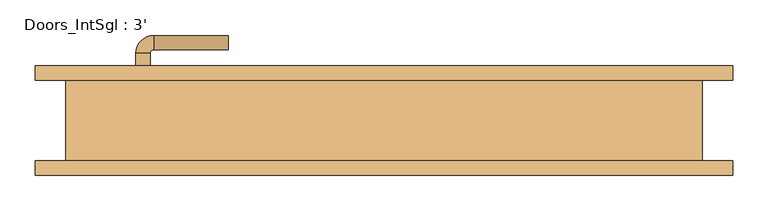
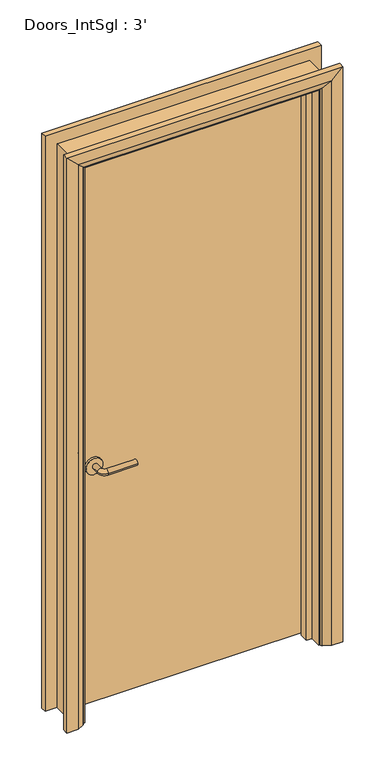
"""IFC4 building model written with IfcOpenShell, lengths in millimetres: door geometry, Doors_IntSgl : 3'."""

from ifc_helpers import new_model, si_unit, point, frame, frame_2d, origin, place, context, project, spatial, polyline, circle_curve, ellipse_curve, trimmed, segment, composite_curve, outline, extrude, faceted_brep, source, transform, mapped, element, save
from ifc_brep_helpers import plane_surface, cylinder_surface, revolved_surface, advanced_brep


def doors_intsgl_3_11801b65(model_context):
    return source(origin(), model_context, "Body", "SolidModel", [
        advanced_brep(
        [(-350.2, 11.15, 900.0), (-330.2, 11.15, 900.0), (-330.2, -18.85, 900.0), (-350.2, -18.85, 900.0), (-325.2, -23.85, 900.0), (-325.2, -43.85, 900.0), (-220.2, -43.85, 900.0), (-220.2, -23.85, 900.0)],
        [
            (0, 1, circle_curve(frame((-340.2, 11.15, 900.0), z_axis=(0.0, 1.0, 0.0), x_axis=(1.0, 0.0, 0.0)), 10.0)),
            (1, 0, circle_curve(frame((-340.2, 11.15, 900.0), z_axis=(0.0, 1.0, 0.0), x_axis=(1.0, 0.0, 0.0)), 10.0)),
            (1, 2),
            (2, 3, circle_curve(frame((-340.2, -18.85, 900.0), z_axis=(0.0, 1.0, 0.0), x_axis=(1.0, 0.0, 0.0)), 10.0)),
            (3, 0),
            (3, 2, circle_curve(frame((-340.2, -18.85, 900.0), z_axis=(0.0, 1.0, 0.0), x_axis=(1.0, 0.0, 0.0)), 10.0)),
            (4, 5, circle_curve(frame((-325.2, -33.85, 900.0), z_axis=(-1.0, 0.0, 0.0), x_axis=(0.0, 1.0, 0.0)), 10.0)),
            (5, 3, circle_curve(frame((-325.2, -18.85, 900.0), z_axis=(0.0, 0.0, -1.0), x_axis=(-1.0, 0.0, 0.0)), 25.0)),
            (2, 4, circle_curve(frame((-325.2, -18.85, 900.0), z_axis=(0.0, 0.0, 1.0), x_axis=(-1.0, 0.0, 0.0)), 5.0)),
            (5, 4, circle_curve(frame((-325.2, -33.85, 900.0), z_axis=(-1.0, 0.0, 0.0), x_axis=(0.0, 1.0, 0.0)), 10.0)),
            (6, 7, circle_curve(frame((-220.2, -33.85, 900.0), z_axis=(1.0, 0.0, 0.0), x_axis=(0.0, 1.0, 0.0)), 10.0)),
            (7, 6, circle_curve(frame((-220.2, -33.85, 900.0), z_axis=(1.0, 0.0, 0.0), x_axis=(0.0, 1.0, 0.0)), 10.0)),
            (4, 7),
            (6, 5),
        ],
        [
            plane_surface(frame((-340.2, 11.15, 900.0), z_axis=(0.0, 1.0, 0.0), x_axis=(0.0, 0.0, 1.0))),
            cylinder_surface(frame((-340.2, 11.15, 900.0), z_axis=(0.0, 1.0, 0.0), x_axis=(1.0, 0.0, 0.0)), 10.0),
            revolved_surface(trimmed(ellipse_curve(frame((-340.2, -18.85, 900.0), z_axis=(0.0, -1.0, 0.0), x_axis=(1.0, 0.0, 0.0)), 10.0, 10.0), [point((-350.2, -18.85, 900.0))], [point((-330.2, -18.85, 900.0))], True, "CARTESIAN"), (-325.2, -18.85, 900.0), (0.0, 0.0, -1.0)),
            revolved_surface(trimmed(ellipse_curve(frame((-340.2, -18.85, 900.0), z_axis=(0.0, -1.0, 0.0), x_axis=(1.0, 0.0, 0.0)), 10.0, 10.0), [point((-330.2, -18.85, 900.0))], [point((-350.2, -18.85, 900.0))], True, "CARTESIAN"), (-325.2, -18.85, 900.0), (0.0, 0.0, -1.0)),
            plane_surface(frame((-220.2, -33.85, 900.0), z_axis=(1.0, 0.0, 0.0), x_axis=(0.0, 0.0, 1.0))),
            cylinder_surface(frame((-325.2, -33.85, 900.0), z_axis=(-1.0, 0.0, 0.0), x_axis=(0.0, 1.0, 0.0)), 10.0),
        ],
        [
            (0, [[1, 2]]),
            (1, [[3, 4, 5, -2]]),
            (1, [[-5, 6, -3, -1]]),
            (2, [[7, 8, -4, 9]]),
            (3, [[10, -9, -6, -8]]),
            (4, [[11, 12]]),
            (5, [[13, -11, 14, -7]]),
            (5, [[-14, -12, -13, -10]]),
        ],
    ),
        extrude(outline(composite_curve([segment(trimmed(circle_curve(frame_2d((900.0, -342.7)), 30.0), [point((900.0, -372.7))], [point((900.0, -312.7))], False, "CARTESIAN"), True, "CONTINUOUS"), segment(trimmed(circle_curve(frame_2d((900.0, -342.7)), 30.0), [point((900.0, -312.7))], [point((900.0, -372.7))], False, "CARTESIAN"), True, "CONTINUOUS")], self_intersect=False)), frame((0.0, 11.15, 0.0), z_axis=(0.0, 1.0, 0.0), x_axis=(0.0, 0.0, 1.0)), (0.0, 0.0, 1.0), 8.0),
        advanced_brep(
        [(-350.2, 65.15, 900.0), (-330.2, 65.15, 900.0), (-350.2, 95.15, 900.0), (-330.2, 95.15, 900.0), (-325.2, 100.15, 900.0), (-325.2, 120.15, 900.0), (-220.2, 120.15, 900.0), (-220.2, 100.15, 900.0)],
        [
            (0, 1, circle_curve(frame((-340.2, 65.15, 900.0), z_axis=(0.0, -1.0, 0.0), x_axis=(1.0, 0.0, 0.0)), 10.0)),
            (1, 0, circle_curve(frame((-340.2, 65.15, 900.0), z_axis=(0.0, -1.0, 0.0), x_axis=(1.0, 0.0, 0.0)), 10.0)),
            (0, 2),
            (2, 3, circle_curve(frame((-340.2, 95.15, 900.0), z_axis=(0.0, -1.0, 0.0), x_axis=(1.0, 0.0, 0.0)), 10.0)),
            (3, 1),
            (3, 2, circle_curve(frame((-340.2, 95.15, 900.0), z_axis=(0.0, -1.0, 0.0), x_axis=(1.0, 0.0, 0.0)), 10.0)),
            (4, 3, circle_curve(frame((-325.2, 95.15, 900.0), z_axis=(0.0, 0.0, 1.0), x_axis=(-1.0, 0.0, 0.0)), 5.0)),
            (2, 5, circle_curve(frame((-325.2, 95.15, 900.0), z_axis=(0.0, 0.0, -1.0), x_axis=(-1.0, 0.0, 0.0)), 25.0)),
            (5, 4, circle_curve(frame((-325.2, 110.15, 900.0), z_axis=(-1.0, 0.0, 0.0), x_axis=(0.0, -1.0, 0.0)), 10.0)),
            (4, 5, circle_curve(frame((-325.2, 110.15, 900.0), z_axis=(-1.0, 0.0, 0.0), x_axis=(0.0, -1.0, 0.0)), 10.0)),
            (6, 7, circle_curve(frame((-220.2, 110.15, 900.0), z_axis=(1.0, 0.0, 0.0), x_axis=(0.0, -1.0, 0.0)), 10.0)),
            (7, 6, circle_curve(frame((-220.2, 110.15, 900.0), z_axis=(1.0, 0.0, 0.0), x_axis=(0.0, -1.0, 0.0)), 10.0)),
            (5, 6),
            (7, 4),
        ],
        [
            plane_surface(frame((-340.2, 65.15, 900.0), z_axis=(0.0, -1.0, 0.0), x_axis=(0.0, 0.0, 1.0))),
            cylinder_surface(frame((-340.2, 65.15, 900.0), z_axis=(0.0, -1.0, 0.0), x_axis=(1.0, 0.0, 0.0)), 10.0),
            revolved_surface(trimmed(ellipse_curve(frame((-340.2, 95.15, 900.0), z_axis=(0.0, -1.0, 0.0), x_axis=(1.0, 0.0, 0.0)), 10.0, 10.0), [point((-350.2, 95.15, 900.0))], [point((-330.2, 95.15, 900.0))], True, "CARTESIAN"), (-325.2, 95.15, 900.0), (0.0, 0.0, -1.0)),
            revolved_surface(trimmed(ellipse_curve(frame((-340.2, 95.15, 900.0), z_axis=(0.0, -1.0, 0.0), x_axis=(1.0, 0.0, 0.0)), 10.0, 10.0), [point((-330.2, 95.15, 900.0))], [point((-350.2, 95.15, 900.0))], True, "CARTESIAN"), (-325.2, 95.15, 900.0), (0.0, 0.0, -1.0)),
            plane_surface(frame((-220.2, 110.15, 900.0), z_axis=(1.0, 0.0, 0.0), x_axis=(0.0, 0.0, 1.0))),
            cylinder_surface(frame((-325.2, 110.15, 900.0), z_axis=(-1.0, 0.0, 0.0), x_axis=(0.0, -1.0, 0.0)), 10.0),
        ],
        [
            (0, [[1, 2]]),
            (1, [[-1, 3, 4, 5]]),
            (1, [[-2, -5, 6, -3]]),
            (2, [[7, -4, 8, 9]]),
            (3, [[-8, -6, -7, 10]]),
            (4, [[11, 12]]),
            (5, [[-9, 13, -12, 14]]),
            (5, [[-10, -14, -11, -13]]),
        ],
    ),
        extrude(outline(composite_curve([segment(trimmed(circle_curve(frame_2d((900.0, -342.7)), 30.0), [point((900.0, -372.7))], [point((900.0, -312.7))], False, "CARTESIAN"), True, "CONTINUOUS"), segment(trimmed(circle_curve(frame_2d((900.0, -342.7)), 30.0), [point((900.0, -312.7))], [point((900.0, -372.7))], False, "CARTESIAN"), True, "CONTINUOUS")], self_intersect=False)), frame((0.0, 57.15, 0.0), z_axis=(0.0, 1.0, 0.0), x_axis=(0.0, 0.0, 1.0)), (0.0, 0.0, 1.0), 8.0),
        extrude(outline(polyline([(415.2, 19.15), (-415.2, 19.15), (-415.2, 57.15), (415.2, 57.15), (415.2, 19.15)])), frame((0.0, 0.0, 8.0), z_axis=(0.0, 0.0, 1.0), x_axis=(1.0, 0.0, 0.0)), (0.0, 0.0, 1.0), 2083.6),
        advanced_brep(
        [(492.2, 77.15, 0.0), (492.2, 57.15, 0.0), (422.2, 57.15, 0.0), (426.2, 63.15, 0.0), (452.2, 77.15, 0.0), (492.2, 77.15, 2168.6), (492.2, 57.15, 2168.6), (-492.2, 57.15, 2168.6), (-492.2, 57.15, 0.0), (-422.2, 57.15, 0.0), (-422.2, 57.15, 2098.6), (422.2, 57.15, 2098.6), (426.2, 63.15, 2102.6), (452.2, 77.15, 2128.6), (-452.2, 77.15, 2128.6), (-452.2, 77.15, 0.0), (-492.2, 77.15, 0.0), (-492.2, 77.15, 2168.6), (-426.2, 63.15, 0.0), (-426.2, 63.15, 2102.6)],
        [
            (0, 1),
            (1, 2),
            (2, 3, circle_curve(frame((430.2, 56.15, 0.0), z_axis=(0.0, 0.0, -1.0), x_axis=(1.0, 0.0, 0.0)), 8.0622577)),
            (3, 4),
            (4, 0),
            (0, 5),
            (5, 6),
            (6, 1),
            (6, 7),
            (7, 8),
            (8, 9),
            (9, 10),
            (10, 11),
            (11, 2),
            (11, 12, ellipse_curve(frame((430.2, 56.15, 2106.6), z_axis=(0.7071067811865475, 0.0, -0.7071067811865475), x_axis=(-0.7071067811865474, 0.0, -0.7071067811865476)), 11.4017543, 8.0622577)),
            (12, 3),
            (12, 13),
            (13, 4),
            (13, 14),
            (14, 15),
            (15, 16),
            (16, 17),
            (17, 5),
            (7, 17),
            (16, 8),
            (15, 18),
            (18, 9, circle_curve(frame((-430.2, 56.15, 0.0), z_axis=(0.0, 0.0, -1.0), x_axis=(-1.0, 0.0, 0.0)), 8.0622577)),
            (19, 10, ellipse_curve(frame((-430.2, 56.15, 2106.6), z_axis=(-0.7071067811865475, 0.0, -0.7071067811865475), x_axis=(-0.7071067811865474, 0.0, 0.7071067811865476)), 11.4017543, 8.0622577)),
            (18, 19),
            (14, 19),
            (19, 12),
        ],
        [
            plane_surface(frame((422.2, 57.15, 0.0), z_axis=(0.0, 0.0, -1.0), x_axis=(0.0, -1.0, 0.0))),
            plane_surface(frame((492.2, 77.15, 0.0), z_axis=(1.0, 0.0, 0.0), x_axis=(0.0, 0.0, 1.0))),
            plane_surface(frame((492.2, 57.15, 0.0), z_axis=(0.0, -1.0, 0.0), x_axis=(0.0, 0.0, 1.0))),
            cylinder_surface(frame((430.2, 56.15, 0.0), z_axis=(0.0, 0.0, -1.0), x_axis=(1.0, 0.0, 0.0)), 8.0622577),
            plane_surface(frame((426.2, 63.15, 0.0), z_axis=(-0.4740998230350126, 0.880471099922178, 0.0), x_axis=(0.0, 0.0, 1.0))),
            plane_surface(frame((452.2, 77.15, 0.0), z_axis=(0.0, 1.0, 0.0), x_axis=(0.0, 0.0, 1.0))),
            plane_surface(frame((-492.2, 77.15, 2168.6), z_axis=(-1.0, 0.0, 0.0), x_axis=(0.0, 0.0, -1.0))),
            plane_surface(frame((-422.2, 57.15, 0.0), z_axis=(0.0, 0.0, -1.0), x_axis=(0.0, -1.0, 0.0))),
            cylinder_surface(frame((-430.2, 56.15, 2098.6), z_axis=(0.0, 0.0, 1.0), x_axis=(-1.0, 0.0, 0.0)), 8.0622577),
            plane_surface(frame((-426.2, 63.15, 2102.6), z_axis=(0.47409982303501824, 0.8804710999221749, 0.0), x_axis=(0.0, 0.0, -1.0))),
            plane_surface(frame((492.2, 77.15, 2168.6), z_axis=(0.0, 0.0, 1.0), x_axis=(-1.0, 0.0, 0.0))),
            cylinder_surface(frame((422.2, 56.15, 2106.6), z_axis=(1.0, 0.0, 0.0), x_axis=(0.0, 0.0, 1.0)), 8.0622577),
            plane_surface(frame((426.2, 63.15, 2102.6), z_axis=(0.0, 0.8804710999221764, -0.4740998230350154), x_axis=(-1.0, 0.0, 0.0))),
        ],
        [
            (0, [[1, 2, 3, 4, 5]]),
            (1, [[-1, 6, 7, 8]]),
            (2, [[-2, -8, 9, 10, 11, 12, 13, 14]]),
            (3, [[-3, -14, 15, 16]]),
            (4, [[-4, -16, 17, 18]]),
            (5, [[-5, -18, 19, 20, 21, 22, 23, -6]]),
            (6, [[24, -22, 25, -10]]),
            (7, [[-21, 26, 27, -11, -25]]),
            (8, [[28, -12, -27, 29]]),
            (9, [[30, -29, -26, -20]]),
            (10, [[-7, -23, -24, -9]]),
            (11, [[-15, -13, -28, 31]]),
            (12, [[-17, -31, -30, -19]]),
        ],
    ),
        extrude(outline(polyline([(0.0, -417.2), (0.0, -398.2), (2074.6, -398.2), (2074.6, 398.2), (0.0, 398.2), (0.0, 417.2), (2093.6, 417.2), (2093.6, -417.2), (0.0, -417.2)])), frame((0.0, -14.85, 0.0), z_axis=(0.0, 1.0, 0.0), x_axis=(0.0, 0.0, 1.0)), (0.0, 0.0, 1.0), 32.0),
        advanced_brep(
        [(-492.2, -77.15, 0.0), (-492.2, -57.15, 0.0), (-422.2, -57.15, 0.0), (-426.2, -63.15, 0.0), (-452.2, -77.15, 0.0), (-492.2, -77.15, 2168.6), (-492.2, -57.15, 2168.6), (-422.2, -57.15, 2098.6), (-426.2, -63.15, 2102.6), (-452.2, -77.15, 2128.6), (492.2, -77.15, 0.0), (452.2, -77.15, 0.0), (426.2, -63.15, 0.0), (422.2, -57.15, 0.0), (492.2, -57.15, 0.0), (492.2, -77.15, 2168.6), (452.2, -77.15, 2128.6), (426.2, -63.15, 2102.6), (422.2, -57.15, 2098.6), (492.2, -57.15, 2168.6)],
        [
            (0, 1),
            (1, 2),
            (2, 3, circle_curve(frame((-430.2, -56.15, 0.0), z_axis=(0.0, 0.0, -1.0), x_axis=(-1.0, 0.0, 0.0)), 8.0622577)),
            (3, 4),
            (4, 0),
            (0, 5),
            (5, 6),
            (6, 1),
            (6, 7),
            (7, 2),
            (7, 8, ellipse_curve(frame((-430.2, -56.15, 2106.6), z_axis=(-0.7071067811865475, 0.0, -0.7071067811865475), x_axis=(0.7071067811865474, 0.0, -0.7071067811865476)), 11.4017543, 8.0622577)),
            (8, 3),
            (8, 9),
            (9, 4),
            (9, 5),
            (10, 11),
            (11, 12),
            (12, 13, circle_curve(frame((430.2, -56.15, 0.0), z_axis=(0.0, 0.0, -1.0), x_axis=(1.0, 0.0, 0.0)), 8.0622577)),
            (13, 14),
            (14, 10),
            (15, 16),
            (16, 11),
            (10, 15),
            (16, 17),
            (17, 12),
            (17, 18, ellipse_curve(frame((430.2, -56.15, 2106.6), z_axis=(0.7071067811865475, 0.0, -0.7071067811865475), x_axis=(0.7071067811865474, 0.0, 0.7071067811865476)), 11.4017543, 8.0622577)),
            (18, 13),
            (18, 19),
            (19, 14),
            (19, 15),
            (5, 15),
            (19, 6),
            (18, 7),
            (17, 8),
            (16, 9),
        ],
        [
            plane_surface(frame((-422.2, -129.9510989, 0.0), z_axis=(0.0, 0.0, -1.0), x_axis=(1.0, 0.0, 0.0))),
            plane_surface(frame((-492.2, -77.15, 0.0), z_axis=(-1.0, 0.0, 0.0), x_axis=(0.0, 0.0, 1.0))),
            plane_surface(frame((-492.2, -57.15, 0.0), z_axis=(0.0, 1.0, 0.0), x_axis=(0.0, 0.0, 1.0))),
            cylinder_surface(frame((-430.2, -56.15, 0.0), z_axis=(0.0, 0.0, -1.0), x_axis=(-1.0, 0.0, 0.0)), 8.0622577),
            plane_surface(frame((-426.2, -63.15, 0.0), z_axis=(0.4740998230350183, -0.8804710999221749, 0.0), x_axis=(0.0, 0.0, 1.0))),
            plane_surface(frame((-452.2, -77.15, 0.0), z_axis=(0.0, -1.0, 0.0), x_axis=(0.0, 0.0, 1.0))),
            plane_surface(frame((422.2, -129.9510989, 0.0), z_axis=(0.0, 0.0, -1.0), x_axis=(-1.0, 0.0, 0.0))),
            plane_surface(frame((452.2, -77.15, 2128.6), z_axis=(0.0, -1.0, 0.0), x_axis=(0.0, 0.0, -1.0))),
            plane_surface(frame((426.2, -63.15, 2102.6), z_axis=(-0.4740998230350183, -0.8804710999221749, 0.0), x_axis=(0.0, 0.0, -1.0))),
            cylinder_surface(frame((430.2, -56.15, 2098.6), z_axis=(0.0, 0.0, 1.0), x_axis=(1.0, 0.0, 0.0)), 8.0622577),
            plane_surface(frame((492.2, -57.15, 2168.6), z_axis=(0.0, 1.0, 0.0), x_axis=(0.0, 0.0, -1.0))),
            plane_surface(frame((492.2, -77.15, 2168.6), z_axis=(1.0, 0.0, 0.0), x_axis=(0.0, 0.0, -1.0))),
            plane_surface(frame((-492.2, -77.15, 2168.6), z_axis=(0.0, 0.0, 1.0), x_axis=(1.0, 0.0, 0.0))),
            plane_surface(frame((-492.2, -57.15, 2168.6), z_axis=(0.0, 1.0, 0.0), x_axis=(1.0, 0.0, 0.0))),
            cylinder_surface(frame((-422.2, -56.15, 2106.6), z_axis=(-1.0, 0.0, 0.0), x_axis=(0.0, 0.0, 1.0)), 8.0622577),
            plane_surface(frame((-426.2, -63.15, 2102.6), z_axis=(0.0, -0.8804710999221749, -0.4740998230350183), x_axis=(1.0, 0.0, 0.0))),
            plane_surface(frame((-452.2, -77.15, 2128.6), z_axis=(0.0, -1.0, 0.0), x_axis=(1.0, 0.0, 0.0))),
        ],
        [
            (0, [[1, 2, 3, 4, 5]]),
            (1, [[-1, 6, 7, 8]]),
            (2, [[-2, -8, 9, 10]]),
            (3, [[-3, -10, 11, 12]]),
            (4, [[-4, -12, 13, 14]]),
            (5, [[-5, -14, 15, -6]]),
            (6, [[16, 17, 18, 19, 20]]),
            (7, [[21, 22, -16, 23]]),
            (8, [[24, 25, -17, -22]]),
            (9, [[26, 27, -18, -25]]),
            (10, [[28, 29, -19, -27]]),
            (11, [[30, -23, -20, -29]]),
            (12, [[-7, 31, -30, 32]]),
            (13, [[-9, -32, -28, 33]]),
            (14, [[-11, -33, -26, 34]]),
            (15, [[-13, -34, -24, 35]]),
            (16, [[-15, -35, -21, -31]]),
        ],
    ),
        faceted_brep([(-417.2, 57.15, 0.0), (-417.2, -57.15, 0.0), (-449.2, -57.15, 0.0), (-449.2, 57.15, 0.0), (-417.2, 57.15, 2093.6), (-417.2, -57.15, 2093.6), (-449.2, -57.15, 2125.6), (-449.2, 57.15, 2125.6), (417.2, 57.15, 0.0), (449.2, 57.15, 0.0), (449.2, -57.15, 0.0), (417.2, -57.15, 0.0), (417.2, 57.15, 2093.6), (449.2, 57.15, 2125.6), (449.2, -57.15, 2125.6), (417.2, -57.15, 2093.6)], [[[0, 1, 2, 3]], [[1, 0, 4, 5]], [[2, 1, 5, 6]], [[3, 2, 6, 7]], [[0, 3, 7, 4]], [[8, 9, 10, 11]], [[12, 13, 9, 8]], [[13, 14, 10, 9]], [[14, 15, 11, 10]], [[15, 12, 8, 11]], [[5, 4, 12, 15]], [[6, 5, 15, 14]], [[7, 6, 14, 13]], [[4, 7, 13, 12]]]),
    ])


if __name__ == "__main__":
    model = new_model("IFC4")
    model_context = context("Model", 3, world=origin())
    ifc_project = project(units=[si_unit("LENGTHUNIT", "METRE", prefix="MILLI")], contexts=[model_context])
    site = spatial("IfcSite", under=ifc_project)
    building = spatial("IfcBuilding", under=site)
    placement = place(None, origin())
    doors_intsgl_3_shape = doors_intsgl_3_11801b65(model_context)
    element("IfcDoor", 1, ObjectType="Doors_IntSgl : 3'", at=placement, inside=building, context=model_context, shape_type="MappedRepresentation", body=[
        mapped(doors_intsgl_3_shape, transform((0.0, 0.0, 0.0), x_axis=(1.0, 0.0, 0.0), y_axis=(0.0, 1.0, 0.0), z_axis=(0.0, 0.0, 1.0))),
    ])
    save(model, "model.ifc")

# Revit data of these elements
# Type "Doors_IntSgl : 3'"
#   Type Mark = "47"
#   Type Comments = "Internal Single"
#   Operation = "SingleSwingRight"
#   Manufacturer = "Revit"
#   Keynote = "L20"
#   Description = "Internal Single Door"
#   Analytic Construction = "Metal"
#   UnderCut = 0' - 0.31496"
#   Tolerance = 0' - 0.07874"
#   Thickness = 0' - 1.49606"
#   Thermal Resistance (R) = 0.270117 (m²·K)/W
#   Structural Tolerance = 0' - 0.31496"
#   StopDepth = 0' - 1.25984"
#   Stop Thickness = 0' - 0.74803"
#   Rough Width = 3' - 0"
#   Rough Height = 7' - 0"
#   Height to Top Lock Rail = 3' - 3.37008"
#   Heat Transfer Coefficient (U) = 3.7021 W/(m²·K)
#   Handle Z Distance = 2' - 11.43307"
#   Handle X Distance = 0' - 2.95276"
#   Frame Thickness = 0' - 1.25984"
#   Door Panel Width = 2' - 8.69291"
#   Door Panel Thickness = 0' - 1.49606"
#   Door Panel Offset = 0' - 0"
#   Height = 7' - 0"
#   Width = 3' - 0"
#   Door Panel Height = 6' - 10.0315"
#   Architrave Setback = 0' - 0.19685"
#   Vis - Ironmongery = yes
#   Material Ironmongery = Door - Handle
#   Material Frame = Door - Frame/Mullion (1)
#   Material Door = Door - Panel
#   Material Architrave = Door - Architrave
#   Visual Light Transmittance = 0
#   Solar Heat Gain Coefficient = 0
#   Function = (empty or 0)
#   Wall Closure = (empty or 0)
# Element 1 (IfcDoor, "Doors_IntSgl : 3'")
#   Materials on its faces: "Door - Architrave", "Door - Handle", "Door - Frame/Mullion (1)", "Door - Panel"
# Materials
#   "Door - Handle": colour RGB 0 0 0, transparency 0, Keynote = "P21", Cost = 0
#   "Door - Frame/Mullion (1)": class "Wood", colour RGB 212 179 113, transparency 0, Keynote = "L20", Cost = 0
#   "Door - Panel": class "Wood", colour RGB 210 159 95, transparency 0, Keynote = "L20", Cost = 0
#   "Door - Architrave": class "Wood", colour RGB 154 90 5, transparency 0, Keynote = "P20", Cost = 0
